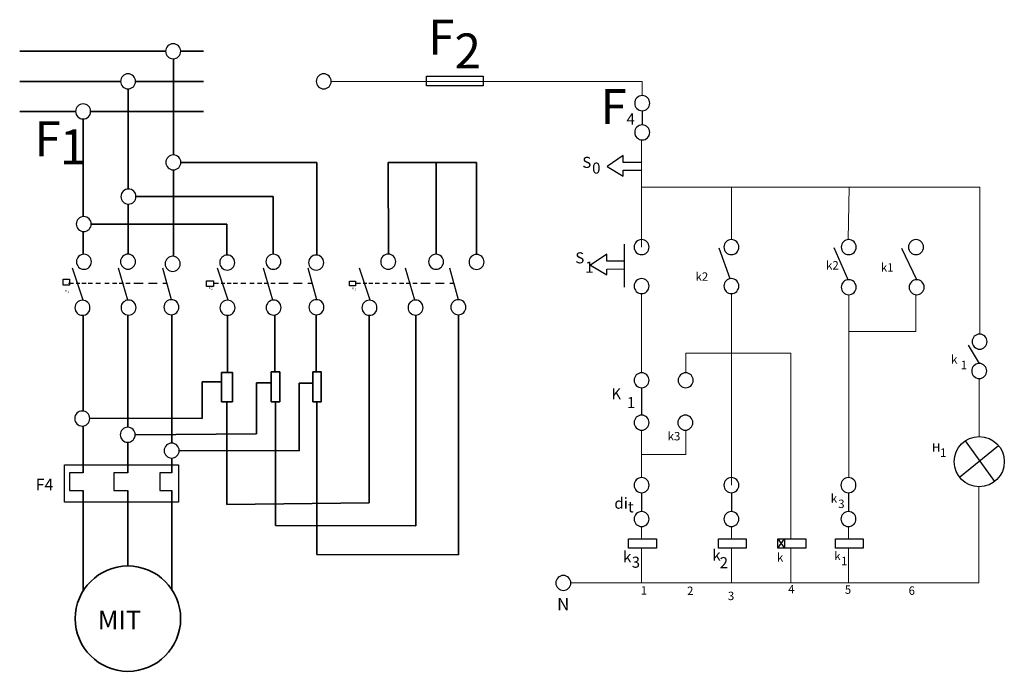
# Model space of a CAD drawing. Units: inches. Extents: x 435 to 1289, y 213 to 521.
# Tile 1 of 1: x 435.3 to 762.6, y 213.4 to 430.1. Entities that reach past the tile are written whole.
import ezdxf

# ---------------------------------------------------------------- set-up
doc = ezdxf.new("R2010")
doc.units = ezdxf.units.IN
doc.header["$MEASUREMENT"] = 0
for name, color, linetype, lineweight in [('E-ANNO-TEXT', 7, 'Continuous', 18), ('E-CTRL-COIL', 3, 'Continuous', 25), ('E-CTRL-CONT', 2, 'Continuous', 25), ('E-CTRL-INDC', 3, 'Continuous', 25), ('E-CTRL-SWCH', 3, 'Continuous', 25), ('E-CTRL-WIRE', 4, 'Continuous', 18), ('E-POWR-CONT', 2, 'Continuous', 25), ('E-POWR-EQPM', 7, 'Continuous', 35), ('E-POWR-WIRE', 7, 'Continuous', 35), ('E-PROT', 1, 'Continuous', 25), ('E-TERM', 7, 'Continuous', 25)]:
    doc.layers.add(name, color=color, linetype=linetype, lineweight=lineweight)
doc.styles.get("Standard").update_dxf_attribs({"font": 'arial.ttf'})

# ---------------------------------------------------------------- blocks, each defined once
blk = doc.blocks.new('CONTACTOR-3P-MOVING-CONTACTS')
for p, q in [((4.85, 4.99), (1.32, 15.73)), ((19.73, 5.05), (16.59, 15.73)), ((34.3, 5.19), (31.42, 15.73)), ((0, 10.66), (1.63, 10.66)), ((2.59, 10.66), (3.77, 10.66)), ((4.5, 10.66), (5.83, 10.66)), ((6.5, 10.66), (8.02, 10.66)), ((9.05, 10.66), (10.7, 10.66)), ((12.09, 10.66), (13.54, 10.66)), ((14.63, 10.66), (16.05, 10.66)), ((16.86, 10.66), (18.3, 10.66)), ((19.08, 10.66), (20.48, 10.66)), ((21.77, 10.66), (24.84, 10.66)), ((26.58, 10.66), (29.45, 10.66)), ((31.39, 10.66), (32.8, 10.66))]:
    blk.add_line(p, q)
for points in [[(2.15, 2.5, 1), (7.15, 2.5, 1)], [(17.48, 2.57, 1), (22.48, 2.57, 1)], [(31.71, 2.7, 1), (36.71, 2.7, 1)]]:
    blk.add_lwpolyline(points, format="xyb", close=True)
blk = doc.blocks.new('CONTROL-CONTACT-CLOSED')
blk.add_line((2.5, 11.27), (2.5, 5))
for points in [[(0, 13.77, 1), (5, 13.77, 1)], [(0, 2.5, 1), (5, 2.5, 1)]]:
    blk.add_lwpolyline(points, format="xyb", close=True)
blk = doc.blocks.new('CONTACTOR-COIL')
blk.add_lwpolyline([(0, 3.11), (9.27, 3.11), (9.27, 0), (0, 0)], close=True)
blk = doc.blocks.new('CONNECTION-NODE')
blk.add_lwpolyline([(0, 2.5, 1), (5, 2.5, 1)], format="xyb", close=True)
blk = doc.blocks.new('POWER-FIXED-CONTACT')
blk.add_lwpolyline([(0, 2.5, 1), (5, 2.5, 1)], format="xyb", close=True)

msp = doc.modelspace()

# ---------------------------------------------------------------- linework, layer by layer
at = {"layer": 'E-CTRL-COIL'}
for p, q in [((687.4, 257.44), (689.62, 254.33)), ((687.4, 254.33), (689.62, 257.44)), ((689.62, 257.44), (689.62, 254.33))]:
    msp.add_line(p, q, dxfattribs=at)
msp.add_lwpolyline([(687.4, 257.44), (696.67, 257.44), (696.67, 254.33), (687.4, 254.33)], close=True, dxfattribs=at)
at = {"layer": 'E-CTRL-CONT'}
for p, q in [((671.46, 343.95), (667.87, 354.13)), ((710.72, 343.62), (706.1, 354.24)), ((733.56, 343.63), (728.6, 354.01)), ((754.44, 315.77), (750.71, 321.91)), ((642.07, 307.68), (642.07, 298.59))]:
    msp.add_line(p, q, dxfattribs=at)
for points in [[(669.41, 354.46, 1), (674.41, 354.46, 1)], [(708.42, 354.46, 1), (713.42, 354.46, 1)], [(730.79, 354.46, 1), (735.79, 354.46, 1)], [(669.41, 341.5, 1), (674.41, 341.5, 1)], [(708.42, 341.13, 1), (713.42, 341.13, 1)], [(731.01, 341.13, 1), (736.01, 341.13, 1)], [(751.94, 323.03, 1), (756.94, 323.03, 1)], [(751.8, 313.27, 1), (756.8, 313.27, 1)], [(639.57, 310.18, 1), (644.57, 310.18, 1)], [(654.22, 310.18, 1), (659.22, 310.18, 1)], [(639.57, 296.09, 1), (644.57, 296.09, 1)], [(654.1, 296.09, 1), (659.1, 296.09, 1)]]:
    msp.add_lwpolyline(points, format="xyb", close=True, dxfattribs=at)
at = {"layer": 'E-CTRL-INDC'}
for p, q in [((747.8, 277.94), (760.66, 288.52)), ((749.66, 290.03), (759.35, 276.49))]:
    msp.add_line(p, q, dxfattribs=at)
msp.add_circle((754.32, 283.12), 8.33, dxfattribs=at)
at = {"layer": 'E-CTRL-SWCH'}
for p, q in [((635.98, 384.93), (630.61, 381.28)), ((635.98, 382.65), (635.98, 384.93)), ((630.61, 381.28), (635.98, 378.08)), ((642.07, 382.65), (635.98, 382.65)), ((635.98, 380.03), (642.07, 380.05)), ((635.98, 378.08), (635.98, 380.03)), ((636.3, 355.47), (636.3, 341.19)), ((630.46, 352.08), (625.09, 348.43)), ((630.46, 349.8), (630.46, 352.08)), ((625.09, 348.43), (630.46, 345.23)), ((636.3, 349.8), (630.46, 349.8)), ((630.46, 347.18), (636.3, 347.2)), ((630.46, 345.23), (630.46, 347.18))]:
    msp.add_line(p, q, dxfattribs=at)
for points in [[(639.57, 354.46, 1), (644.57, 354.46, 1)], [(639.57, 341.5, 1), (644.57, 341.5, 1)]]:
    msp.add_lwpolyline(points, format="xyb", close=True, dxfattribs=at)
at = {"layer": 'E-CTRL-WIRE'}
for p, q in [((538.97, 409.6), (642.27, 409.6)), ((642.27, 409.6), (642.27, 404.84)), ((642.07, 390.13), (642.07, 354.46)), ((642.07, 374.4), (754.47, 374.4)), ((671.9, 356.96), (671.92, 374.4)), ((710.78, 356.95), (711.09, 374.4)), ((754.47, 374.4), (754.47, 325.51)), ((642.07, 339), (642.07, 312.68)), ((671.91, 275.3), (671.91, 339)), ((710.92, 277.8), (710.92, 338.63)), ((733.18, 326.43), (733.25, 338.64)), ((710.92, 326.43), (733.18, 326.43)), ((656.78, 312.68), (656.78, 319.21)), ((656.78, 319.21), (691.73, 319.21)), ((691.73, 319.21), (691.73, 257.44)), ((754.32, 310.77), (754.32, 291.45)), ((642.07, 293.59), (642.07, 277.8)), ((656.72, 285.46), (656.72, 293.59)), ((642.07, 285.46), (656.72, 285.46)), ((691.73, 272.8), (691.73, 266.53)), ((754.16, 274.8), (754.16, 242.78)), ((642.07, 261.53), (642.07, 257.44)), ((671.91, 261.53), (671.91, 257.44)), ((691.73, 261.53), (691.73, 257.44)), ((710.83, 261.53), (710.83, 257.44)), ((642.06, 254.33), (642.06, 242.78)), ((671.9, 254.33), (671.9, 242.78)), ((691.72, 254.33), (691.72, 242.78)), ((710.82, 254.33), (710.82, 242.78)), ((642.06, 242.78), (618.62, 242.78)), ((642.06, 242.78), (754.16, 242.78))]:
    msp.add_line(p, q, dxfattribs=at)
at = {"layer": 'E-POWR-CONT'}
for points in [[(449.78, 343.83), (451.93, 343.83), (451.93, 341.77), (449.78, 341.77)], [(497.42, 343.28), (499.8, 343.28), (499.8, 341.4), (497.42, 341.4)], [(544.94, 343.14), (546.94, 343.14), (546.94, 341.57), (544.94, 341.57)]]:
    msp.add_lwpolyline(points, close=True, dxfattribs=at)
at = {"layer": 'E-POWR-EQPM'}
for points in [[(502.46, 312.77), (506.02, 312.77), (506.02, 303.03), (502.46, 303.03)], [(518.92, 312.97), (521.75, 312.97), (521.75, 303.03), (518.92, 303.03)], [(532.81, 312.97), (535.58, 312.97), (535.58, 303.03), (532.81, 303.03)]]:
    msp.add_lwpolyline(points, close=True, dxfattribs=at)
msp.add_circle((471.3, 230.9), 17.52, dxfattribs=at)
at = {"layer": 'E-POWR-WIRE'}
for p, q in [((435.32, 419.6), (483.91, 419.6)), ((488.91, 419.6), (496.45, 419.6)), ((486.41, 417.1), (486.41, 385.15)), ((435.32, 409.6), (468.91, 409.6)), ((473.91, 409.6), (496.45, 409.6)), ((471.41, 407.1), (471.41, 373.78)), ((435.32, 399.6), (453.91, 399.6)), ((458.91, 399.6), (496.45, 399.6)), ((456.41, 397.1), (456.41, 364.62)), ((486.41, 380.16), (486.41, 351.4)), ((488.97, 382.65), (534.1, 382.65)), ((534.1, 351.83), (534.1, 382.65)), ((557.81, 382.65), (587.21, 382.65)), ((557.81, 382.65), (557.89, 352.14)), ((573.79, 382.65), (573.8, 352.1)), ((587.21, 382.65), (587.21, 352.03)), ((474.06, 371.28), (519.61, 371.28)), ((519.61, 352.1), (519.61, 371.28)), ((471.41, 368.79), (471.41, 352.14)), ((459.18, 362.14), (504.23, 362.14)), ((504.23, 351.83), (504.23, 362.14)), ((456.41, 359.65), (456.41, 359)), ((456.41, 359), (456.41, 352.07)), ((456.41, 331.8), (456.41, 299.95)), ((471.3, 331.86), (471.3, 294.56)), ((485.91, 331.99), (485.91, 289.29)), ((504.39, 331.79), (504.39, 313.09)), ((520.13, 331.89), (520.13, 313.09)), ((533.84, 331.99), (533.84, 313.09)), ((551.5, 331.79), (551.5, 269.41)), ((567, 331.85), (567, 261.77)), ((581.24, 331.99), (581.24, 252.09)), ((502.46, 309.68), (495.97, 309.68)), ((495.97, 309.68), (495.97, 297.46)), ((518.92, 309.38), (513.99, 309.38)), ((513.99, 309.38), (513.99, 292.35)), ((532.81, 309.19), (528.24, 309.19)), ((528.24, 309.19), (528.24, 286.77)), ((504.14, 303.03), (504.14, 268.83)), ((520.32, 303.03), (520.32, 261.84)), ((534.08, 303.03), (534.08, 252.27)), ((456.41, 294.97), (456.41, 279.35)), ((495.97, 297.46), (458.68, 297.63)), ((513.99, 292.35), (473.8, 292.08)), ((471.3, 289.56), (471.3, 279.35)), ((528.24, 286.77), (488.41, 286.79)), ((485.91, 284.29), (485.91, 279.35)), ((456.41, 273.55), (456.41, 240.13)), ((471.3, 273.55), (471.3, 248.42)), ((485.91, 273.55), (485.91, 240.57)), ((504.14, 268.83), (551.5, 269.41)), ((520.32, 261.84), (567, 261.77)), ((534.08, 252.27), (581.24, 252.09))]:
    msp.add_line(p, q, dxfattribs=at)
at = {"layer": 'E-PROT'}
for p, q in [((642.28, 399.84), (642.28, 395.12)), ((456.41, 279.35), (451.84, 279.35)), ((451.84, 279.35), (451.84, 273.55)), ((471.3, 279.35), (466.65, 279.35)), ((466.65, 279.35), (466.65, 273.55)), ((485.91, 279.35), (481.85, 279.35)), ((481.85, 279.35), (481.85, 273.55)), ((451.84, 273.55), (456.41, 273.55)), ((466.65, 273.55), (471.3, 273.55)), ((481.85, 273.55), (485.91, 273.55))]:
    msp.add_line(p, q, dxfattribs=at)
for points in [[(570.55, 411.29), (589.41, 411.29), (589.41, 408.1), (570.55, 408.1)], [(450.17, 282.04), (488.13, 282.04), (488.13, 269.66), (450.17, 269.66)]]:
    msp.add_lwpolyline(points, close=True, dxfattribs=at)
for points in [[(639.77, 402.34, 1), (644.77, 402.34, 1)], [(639.77, 392.62, 1), (644.77, 392.62, 1)]]:
    msp.add_lwpolyline(points, format="xyb", close=True, dxfattribs=at)

# ---------------------------------------------------------------- block references
at = {"layer": 'E-CTRL-COIL'}
for p in [(637.74, 254.33), (667.58, 254.33), (706.5, 254.33)]:
    msp.add_blockref('CONTACTOR-COIL', p, dxfattribs=at)
at = {"layer": 'E-CTRL-CONT'}
for p in [(639.57, 261.53), (669.41, 261.53), (708.33, 261.53)]:
    msp.add_blockref('CONTROL-CONTACT-CLOSED', p, dxfattribs=at)
at = {"layer": 'E-POWR-CONT'}
for name, p in [('POWER-FIXED-CONTACT', (454.18, 347.09)), ('CONTACTOR-3P-MOVING-CONTACTS', (451.53, 331.79)), ('CONTACTOR-3P-MOVING-CONTACTS', (499.75, 331.79)), ('CONTACTOR-3P-MOVING-CONTACTS', (546.94, 331.79))]:
    msp.add_blockref(name, p, dxfattribs=at)
at = {"layer": 'E-POWR-CONT', "rotation": 180}
for p in [(473.82, 352.14), (488.67, 351.41), (506.82, 351.83), (522.15, 352.1), (536.38, 351.83), (560.32, 352.14), (576.23, 352.1), (589.7, 352.03)]:
    msp.add_blockref('POWER-FIXED-CONTACT', p, dxfattribs=at)
at = {"layer": 'E-TERM', "rotation": 180}
for p in [(488.84, 422.1), (473.84, 412.1), (538.89, 412.1), (488.9, 385.15), (473.98, 373.78), (459.11, 364.64), (458.61, 299.96), (473.73, 294.56), (488.34, 289.29), (618.55, 245.28)]:
    msp.add_blockref('CONNECTION-NODE', p, dxfattribs=at)
at = {"layer": 'E-TERM'}
msp.add_blockref('CONNECTION-NODE', (453.91, 397.1), dxfattribs=at)

# ---------------------------------------------------------------- texts
at = {"layer": 'E-ANNO-TEXT'}
for s, height, p in [('F', 11.64, (571.09, 418.47)), ('2', 11.64, (579.84, 413.88)), ('F', 11.64, (628.4, 395.38)), ('F', 11.64, (440.22, 384.68)), ('4', 3.68, (637.04, 395.24)), ('1', 11.64, (448.67, 381.98)), ('S', 3.68, (622.34, 380.81)), ('0', 3.68, (625.61, 378.91)), ('S', 3.68, (620.02, 349.07)), ('1', 3.68, (623.3, 345.97)), ('k2', 2.804, (703.38, 347.02)), ('k1', 2.804, (721.59, 346.32)), ('k2', 2.804, (659.99, 343.26)), ('K', 0.728, (498.12, 340.52)), ('2', 0.728, (498.95, 340.24)), ('K', 0.728, (545.85, 340.41)), ('3', 0.728, (546.59, 340.09)), ('K', 0.728, (450.39, 339.52)), ('1', 0.728, (451.15, 339.24)), ('k', 2.8, (744.93, 315.73)), ('1', 2.8, (748.15, 313.86)), ('K', 3.68, (632, 303.82)), ('1', 3.68, (637.16, 300.91)), ('k3', 2.804, (650.72, 290.19)), ('H', 2.8, (738.6, 286.46)), ('1', 2.8, (741.27, 284.72)), ('F4', 3.876, (440.64, 273.53)), ('k', 2.8, (704.95, 269.5)), ('di ', 3.679, (633.01, 267.46)), ('t', 3.68, (637.54, 266.24)), ('3', 2.8, (707.42, 267.69)), ('k', 3.68, (635.89, 249.64)), ('k', 3.68, (665.58, 250.21)), ('k', 2.8, (687.05, 249.87)), ('k', 2.8, (706.11, 250.38)), ('3', 3.68, (638.76, 247.84)), ('2', 3.68, (668, 247.68)), ('1', 2.8, (708.4, 248.67)), ('1', 2.8, (641.78, 238.9)), ('2', 2.8, (657.19, 238.76)), ('3', 2.8, (670.75, 237.07)), ('4', 2.8, (690.82, 239.33)), ('5', 2.8, (709.62, 239.18)), ('6', 2.8, (730.82, 238.83)), ('N', 4.13, (613.97, 233.67)), ('MIT', 6.207, (461.28, 227.4))]:
    msp.add_text(s, height=height, dxfattribs=at).set_placement(p)

doc.saveas('drawing.dxf')
